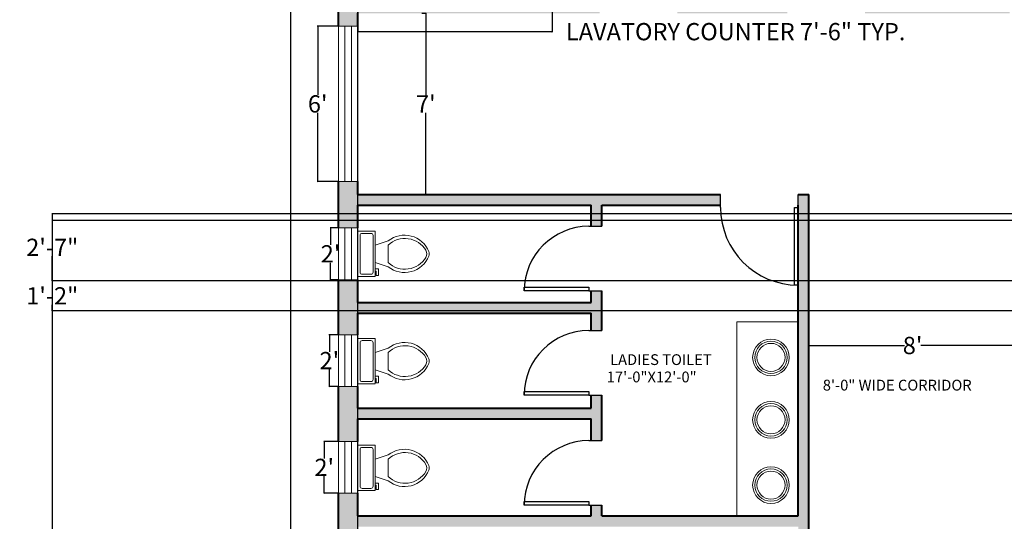
# Model space of a CAD drawing. Units: inches. Extents: x -405 to 940, y 226 to 2032.
# Tile 5 of 10: x -405 to 51, y 1458 to 1691. Entities that reach past the tile are written whole.
import ezdxf

# ---------------------------------------------------------------- set-up
doc = ezdxf.new("R2010")
doc.units = ezdxf.units.IN
doc.header["$MEASUREMENT"] = 0
doc.linetypes.add('ACAD_ISO02W100', pattern=[15, 12, -3])
for name, color, linetype, lineweight in [('A-ANNO-DIMS', 120, 'Continuous', 18), ('A-AREA-IDEN', 32, 'Continuous', 18), ('A-FLOR-FIXT', 175, 'Continuous', 18), ('A-GLAZ-HIDN', 1, 'ACAD_ISO02W100', 18), ('A-WALL-PATT', 8, 'Continuous', 13), ('door', 6, 'Continuous', 25), ('wall', 3, 'Continuous', 40), ('window', 1, 'Continuous', 18)]:
    doc.layers.add(name, color=color, linetype=linetype, lineweight=lineweight)
doc.styles.get("Standard").update_dxf_attribs({"font": 'arial.ttf'})
doc.dimstyles.get("Standard").update_dxf_attribs({"dimtxt": 8, "dimasz": 0.18, "dimexe": 0.18, "dimexo": 0.0625, "dimgap": 0.09, "dimtad": 0, "dimtih": 1, "dimtoh": 1, "dimdec": 0, "dimzin": 0, "dimdsep": 46, "dimlunit": 3, "dimtxsty": 'Standard', "dimblk": 'OBLIQUE', "dimcen": 0.09, "dimadec": 0, "dimazin": 0, "dimtfac": 1, "dimtdec": 0, "dimtofl": 0, "dimtmove": 0, "dimatfit": 3, "dimfxl": 1, "dimtolj": 1, "dimtzin": 0, "dimarcsym": 0})

# ---------------------------------------------------------------- blocks, each defined once
blk = doc.blocks.new('*U3')
for p, q in [((0, 0), (0, -6)), ((30, 0), (30, -6))]:
    blk.add_line(p, q)
blk.add_lwpolyline([(0, 0), (0, 30), (1.75, 30), (1.75, 0)], close=True)
blk.add_arc((0, 0), 30, 0, 90)
blk = doc.blocks.new('*U4')
for p, q in [((0, 0), (0, -6)), ((36, 0), (36, -6))]:
    blk.add_line(p, q)
blk.add_lwpolyline([(0, 0), (0, 36), (1.75, 36), (1.75, 0)], close=True)
blk.add_arc((0, 0), 36, 0, 90)
blk = doc.blocks.new('*U6')
for p, q in [((9.5, -6), (9.5, -2)), ((-10, -8.5), (-8, -8.5)), ((-10, -9.5), (-10, -8.5)), ((-8, -8.5), (-8, -8)), ((-7, -8), (-7, -9.5)), ((-4, -8), (-6, -14)), ((4, -8), (6, -14)), ((-7, -9.5), (-10, -9.5)), ((4, -14), (-4, -14))]:
    blk.add_line(p, q)
blk.add_lwpolyline([(10.5, -8), (10.5, 0), (-10.5, 0), (-10.5, -8)], close=True)
for points in [[(-9.5, -2), (-9.5, -6)], [(8.5, -1), (-8.5, -1)], [(-8.5, -7), (8.5, -7)]]:
    blk.add_lwpolyline(points)
for centre, radius, start, end in [((-8.62, -1.88), 0.884, 81.8699, 188.1301), ((8.62, -1.88), 0.884, 351.8699, 98.1301), ((-8.62, -6.12), 0.884, 171.8699, 278.1301), ((8.62, -6.12), 0.884, 261.8699, 8.1301), ((3.52, -21.58), 12.17, 141.4691, 247.9714), ((4.2, -21.82), 11.33, 136.3677, 238.9468), ((-3.52, -21.58), 12.17, 292.0284, 38.5307), ((-4.2, -21.82), 11.33, 301.053, 43.6321), ((0, -27.88), 4, 245.7318, 294.2682), ((0, -29), 4, 254.8605, 285.1395)]:
    blk.add_arc(centre, radius, start, end)
blk = doc.blocks.new('_Oblique')
at = {"color": 0, "linetype": 'ByBlock', "lineweight": -2}
blk.add_line((-0.5, -0.5), (0.5, 0.5), dxfattribs=at)
blk = doc.blocks.new('*D40')
at = {"layer": 'A-ANNO-DIMS', "color": 0, "lineweight": -2, "transparency": 16777216}
for p, q in [((-39.23, 1543.59), (-39.23, 1539.64)), ((56.77, 1543.59), (56.77, 1539.64)), ((-39.23, 1539.82), (4.99, 1539.82)), ((56.77, 1539.82), (12.54, 1539.82))]:
    blk.add_line(p, q, dxfattribs=at)
at = {"layer": 'Defpoints', "color": 0, "transparency": 16777216}
for p in [(-39.23, 1543.65), (56.77, 1543.65), (56.77, 1539.82)]:
    blk.add_point(p, dxfattribs=at)
at = {"layer": 'A-ANNO-DIMS', "color": 0, "lineweight": -2, "transparency": 16777216, "xscale": 0.18, "yscale": 0.18, "zscale": 0.18, "rotation": 180}
blk.add_blockref('_Oblique', (-39.23, 1539.82), dxfattribs=at)
at = {"layer": 'A-ANNO-DIMS', "color": 0, "lineweight": -2, "transparency": 16777216, "xscale": 0.18, "yscale": 0.18, "zscale": 0.18}
blk.add_blockref('_Oblique', (56.77, 1539.82), dxfattribs=at)
at = {"layer": 'A-ANNO-DIMS', "color": 0, "transparency": 16777216, "insert": (8.77, 1539.82), "char_height": 8, "attachment_point": 5}
blk.add_mtext("\\A1;8'", dxfattribs=at)
blk = doc.blocks.new('*D44')
at = {"layer": 'A-ANNO-DIMS', "color": 0, "lineweight": -2, "transparency": 16777216}
for p, q in [((-257.29, 1887.81), (-279.61, 1887.81)), ((-279.43, 1887.81), (-279.43, 1210.99)), ((-279.43, 525.81), (-279.43, 1202.63)), ((-257.29, 525.81), (-279.61, 525.81))]:
    blk.add_line(p, q, dxfattribs=at)
at = {"layer": 'Defpoints', "color": 0, "transparency": 16777216}
for p in [(-257.23, 1887.81), (-279.43, 525.81), (-257.23, 525.81)]:
    blk.add_point(p, dxfattribs=at)
at = {"layer": 'A-ANNO-DIMS', "color": 0, "lineweight": -2, "transparency": 16777216, "xscale": 0.18, "yscale": 0.18, "zscale": 0.18}
for p, rotation in [((-279.43, 1887.81), 90), ((-279.43, 525.81), 270)]:
    blk.add_blockref('_Oblique', p, dxfattribs=dict(at, rotation=rotation))
at = {"layer": 'A-ANNO-DIMS', "color": 0, "transparency": 16777216, "insert": (-279.43, 1206.81), "char_height": 8, "attachment_point": 5}
blk.add_mtext('\\A1;113\'-6"', dxfattribs=at)
blk = doc.blocks.new('*D56')
at = {"layer": 'A-ANNO-DIMS', "color": 0, "lineweight": -2, "transparency": 16777216}
for p, q in [((-257.29, 1495.31), (-264.03, 1495.31)), ((-263.85, 1495.31), (-263.85, 1487.42)), ((-263.85, 1471.31), (-263.85, 1479.2)), ((-257.29, 1471.31), (-264.03, 1471.31))]:
    blk.add_line(p, q, dxfattribs=at)
at = {"layer": 'Defpoints', "color": 0, "transparency": 16777216}
for p in [(-263.85, 1495.31), (-257.23, 1495.31), (-257.23, 1471.31)]:
    blk.add_point(p, dxfattribs=at)
at = {"layer": 'A-ANNO-DIMS', "color": 0, "lineweight": -2, "transparency": 16777216, "xscale": 0.18, "yscale": 0.18, "zscale": 0.18}
for p, rotation in [((-263.85, 1495.31), 90), ((-263.85, 1471.31), 270)]:
    blk.add_blockref('_Oblique', p, dxfattribs=dict(at, rotation=rotation))
at = {"layer": 'A-ANNO-DIMS', "color": 0, "transparency": 16777216, "insert": (-263.85, 1483.31), "char_height": 8, "attachment_point": 5}
blk.add_mtext("\\A1;2'", dxfattribs=at)
blk = doc.blocks.new('*D57')
at = {"layer": 'A-ANNO-DIMS', "color": 0, "lineweight": -2, "transparency": 16777216}
for p, q in [((-257.29, 1544.81), (-261.65, 1544.81)), ((-261.47, 1544.81), (-261.47, 1536.92)), ((-261.47, 1520.81), (-261.47, 1528.7)), ((-257.29, 1520.81), (-261.65, 1520.81))]:
    blk.add_line(p, q, dxfattribs=at)
at = {"layer": 'Defpoints', "color": 0, "transparency": 16777216}
for p in [(-261.47, 1544.81), (-257.23, 1544.81), (-257.23, 1520.81)]:
    blk.add_point(p, dxfattribs=at)
at = {"layer": 'A-ANNO-DIMS', "color": 0, "lineweight": -2, "transparency": 16777216, "xscale": 0.18, "yscale": 0.18, "zscale": 0.18}
for p, rotation in [((-261.47, 1544.81), 90), ((-261.47, 1520.81), 270)]:
    blk.add_blockref('_Oblique', p, dxfattribs=dict(at, rotation=rotation))
at = {"layer": 'A-ANNO-DIMS', "color": 0, "transparency": 16777216, "insert": (-261.47, 1532.81), "char_height": 8, "attachment_point": 5}
blk.add_mtext("\\A1;2'", dxfattribs=at)
blk = doc.blocks.new('*D58')
at = {"layer": 'A-ANNO-DIMS', "color": 0, "lineweight": -2, "transparency": 16777216}
for p, q in [((-257.29, 1594.31), (-261.11, 1594.31)), ((-260.93, 1594.31), (-260.93, 1586.42)), ((-260.93, 1570.31), (-260.93, 1578.2)), ((-257.29, 1570.31), (-261.11, 1570.31))]:
    blk.add_line(p, q, dxfattribs=at)
at = {"layer": 'Defpoints', "color": 0, "transparency": 16777216}
for p in [(-260.93, 1594.31), (-257.23, 1594.31), (-257.23, 1570.31)]:
    blk.add_point(p, dxfattribs=at)
at = {"layer": 'A-ANNO-DIMS', "color": 0, "lineweight": -2, "transparency": 16777216, "xscale": 0.18, "yscale": 0.18, "zscale": 0.18}
for p, rotation in [((-260.93, 1594.31), 90), ((-260.93, 1570.31), 270)]:
    blk.add_blockref('_Oblique', p, dxfattribs=dict(at, rotation=rotation))
at = {"layer": 'A-ANNO-DIMS', "color": 0, "transparency": 16777216, "insert": (-260.93, 1582.31), "char_height": 8, "attachment_point": 5}
blk.add_mtext("\\A1;2'", dxfattribs=at)
blk = doc.blocks.new('*D59')
at = {"layer": 'A-ANNO-DIMS', "color": 0, "lineweight": -2, "transparency": 16777216}
for p, q in [((-218.67, 1693.81), (-216.61, 1693.81)), ((-216.79, 1693.81), (-216.79, 1655.9)), ((-216.79, 1609.81), (-216.79, 1647.72)), ((-218.67, 1609.81), (-216.61, 1609.81))]:
    blk.add_line(p, q, dxfattribs=at)
at = {"layer": 'Defpoints', "color": 0, "transparency": 16777216}
for p in [(-218.73, 1693.81), (-218.73, 1609.81), (-216.79, 1609.81)]:
    blk.add_point(p, dxfattribs=at)
at = {"layer": 'A-ANNO-DIMS', "color": 0, "lineweight": -2, "transparency": 16777216, "xscale": 0.18, "yscale": 0.18, "zscale": 0.18}
for p, rotation in [((-216.79, 1693.81), 90), ((-216.79, 1609.81), 270)]:
    blk.add_blockref('_Oblique', p, dxfattribs=dict(at, rotation=rotation))
at = {"layer": 'A-ANNO-DIMS', "color": 0, "transparency": 16777216, "insert": (-216.79, 1651.81), "char_height": 8, "attachment_point": 5}
blk.add_mtext("\\A1;7'", dxfattribs=at)
blk = doc.blocks.new('*D60')
at = {"layer": 'A-ANNO-DIMS', "color": 0, "lineweight": -2, "transparency": 16777216}
for p, q in [((-257.29, 1687.81), (-267.07, 1687.81)), ((-266.89, 1687.81), (-266.89, 1655.98)), ((-266.89, 1615.81), (-266.89, 1647.64)), ((-257.29, 1615.81), (-267.07, 1615.81))]:
    blk.add_line(p, q, dxfattribs=at)
at = {"layer": 'Defpoints', "color": 0, "transparency": 16777216}
for p in [(-266.89, 1687.81), (-257.23, 1687.81), (-257.23, 1615.81)]:
    blk.add_point(p, dxfattribs=at)
at = {"layer": 'A-ANNO-DIMS', "color": 0, "lineweight": -2, "transparency": 16777216, "xscale": 0.18, "yscale": 0.18, "zscale": 0.18}
for p, rotation in [((-266.89, 1687.81), 90), ((-266.89, 1615.81), 270)]:
    blk.add_blockref('_Oblique', p, dxfattribs=dict(at, rotation=rotation))
at = {"layer": 'A-ANNO-DIMS', "color": 0, "transparency": 16777216, "insert": (-266.89, 1651.81), "char_height": 8, "attachment_point": 5}
blk.add_mtext("\\A1;6'", dxfattribs=at)
blk = doc.blocks.new('LAVATORY-COUNTER-TRIPLE')
for p, q in [((0, 28.51), (89.99, 28.51)), ((89.99, 28.51), (89.99, 0))]:
    blk.add_line(p, q)
for centre, radius in [((14.28, 12.62), 8.5), ((14.28, 12.62), 7.5), ((14.28, 12.62), 6.5), ((44.55, 12.62), 8.5), ((44.55, 12.62), 7.5), ((44.55, 12.62), 6.5), ((73.49, 12.62), 8.5), ((73.49, 12.62), 7.5), ((73.49, 12.62), 6.5)]:
    blk.add_circle(centre, radius)
blk = doc.blocks.new('WIN-PANE-24IN')
for p, q in [((0, 3), (24, 3)), ((0, 0), (24, 0))]:
    blk.add_line(p, q)
blk = doc.blocks.new('WIN-PANE-72IN')
for p, q in [((0, 3), (72, 3)), ((0, 0), (72, 0))]:
    blk.add_line(p, q)
blk = doc.blocks.new('*D93')
at = {"layer": 'A-ANNO-DIMS', "color": 0, "lineweight": -2, "transparency": 16777216}
for p, q in [((-248.23, 1698.75), (-248.23, 1685.13)), ((-158.24, 1698.75), (-158.24, 1685.13)), ((-248.23, 1685.31), (-158.24, 1685.31)), ((-158.24, 1685.31), (-158.06, 1685.31))]:
    blk.add_line(p, q, dxfattribs=at)
at = {"layer": 'Defpoints', "color": 0, "transparency": 16777216}
for p in [(-248.23, 1698.81), (-158.24, 1698.81), (-158.24, 1685.31)]:
    blk.add_point(p, dxfattribs=at)
at = {"layer": 'A-ANNO-DIMS', "color": 0, "lineweight": -2, "transparency": 16777216, "xscale": 0.18, "yscale": 0.18, "zscale": 0.18, "rotation": 180}
blk.add_blockref('_Oblique', (-248.23, 1685.31), dxfattribs=at)
at = {"layer": 'A-ANNO-DIMS', "color": 0, "lineweight": -2, "transparency": 16777216, "xscale": 0.18, "yscale": 0.18, "zscale": 0.18}
blk.add_blockref('_Oblique', (-158.24, 1685.31), dxfattribs=at)
at = {"layer": 'A-ANNO-DIMS', "color": 0, "transparency": 16777216, "insert": (-73.22, 1685.31), "char_height": 8, "attachment_point": 5}
blk.add_mtext('\\A1;LAVATORY COUNTER 7\'-6" TYP.', dxfattribs=at)
blk = doc.blocks.new('*D100')
at = {"layer": 'A-ANNO-DIMS', "color": 0, "lineweight": -2, "transparency": 16777216}
for p, q in [((626.71, 1569.84), (-390.06, 1569.84)), ((-389.88, 1569.84), (-389.88, 1566.93)), ((626.71, 1555.81), (-390.06, 1555.81)), ((-389.88, 1555.81), (-389.88, 1558.72))]:
    blk.add_line(p, q, dxfattribs=at)
at = {"layer": 'Defpoints', "color": 0, "transparency": 16777216}
for p in [(626.77, 1569.84), (-389.88, 1555.81), (626.77, 1555.81)]:
    blk.add_point(p, dxfattribs=at)
at = {"layer": 'A-ANNO-DIMS', "color": 0, "lineweight": -2, "transparency": 16777216, "xscale": 0.18, "yscale": 0.18, "zscale": 0.18}
for p, rotation in [((-389.88, 1569.84), 90), ((-389.88, 1555.81), 270)]:
    blk.add_blockref('_Oblique', p, dxfattribs=dict(at, rotation=rotation))
at = {"layer": 'A-ANNO-DIMS', "color": 0, "transparency": 16777216, "insert": (-389.88, 1562.83), "char_height": 8, "attachment_point": 5}
blk.add_mtext('\\A1;1\'-2"', dxfattribs=at)
blk = doc.blocks.new('*D105')
at = {"layer": 'A-ANNO-DIMS', "color": 0, "lineweight": -2, "transparency": 16777216}
for p, q in [((602.71, 1600.81), (-390.06, 1600.81)), ((-389.88, 1600.81), (-389.88, 1589.43)), ((-389.88, 1569.84), (-389.88, 1581.22)), ((626.71, 1569.84), (-390.06, 1569.84))]:
    blk.add_line(p, q, dxfattribs=at)
at = {"layer": 'Defpoints', "color": 0, "transparency": 16777216}
for p in [(602.77, 1600.81), (-389.88, 1569.84), (626.77, 1569.84)]:
    blk.add_point(p, dxfattribs=at)
at = {"layer": 'A-ANNO-DIMS', "color": 0, "lineweight": -2, "transparency": 16777216, "xscale": 0.18, "yscale": 0.18, "zscale": 0.18}
for p, rotation in [((-389.88, 1600.81), 90), ((-389.88, 1569.84), 270)]:
    blk.add_blockref('_Oblique', p, dxfattribs=dict(at, rotation=rotation))
at = {"layer": 'A-ANNO-DIMS', "color": 0, "transparency": 16777216, "insert": (-389.88, 1585.33), "char_height": 8, "attachment_point": 5}
blk.add_mtext('\\A1;2\'-7"', dxfattribs=at)
blk = doc.blocks.new('*D107')
at = {"layer": 'A-ANNO-DIMS', "color": 0, "lineweight": -2, "transparency": 16777216}
for p, q in [((501.71, 1597.81), (-390.06, 1597.81)), ((-389.88, 1597.81), (-389.88, 1228.98)), ((-389.88, 851.81), (-389.88, 1220.64)), ((501.71, 851.81), (-390.06, 851.81))]:
    blk.add_line(p, q, dxfattribs=at)
at = {"layer": 'Defpoints', "color": 0, "transparency": 16777216}
for p in [(-389.88, 1597.81), (501.77, 1597.81), (501.77, 851.81)]:
    blk.add_point(p, dxfattribs=at)
at = {"layer": 'A-ANNO-DIMS', "color": 0, "lineweight": -2, "transparency": 16777216, "xscale": 0.18, "yscale": 0.18, "zscale": 0.18}
for p, rotation in [((-389.88, 1597.81), 90), ((-389.88, 851.81), 270)]:
    blk.add_blockref('_Oblique', p, dxfattribs=dict(at, rotation=rotation))
at = {"layer": 'A-ANNO-DIMS', "color": 0, "transparency": 16777216, "insert": (-389.88, 1224.81), "char_height": 8, "attachment_point": 5}
blk.add_mtext('\\A1;62\'-2"', dxfattribs=at)
blk = doc.blocks.new('*D109')
at = {"layer": 'A-ANNO-DIMS', "color": 0, "lineweight": -2, "transparency": 16777216}
for p, q in [((-248.23, 750.87), (-248.23, 2020.64)), ((-248.23, 2020.46), (-49.06, 2020.46)), ((177.77, 2020.46), (-21.4, 2020.46)), ((177.77, 750.87), (177.77, 2020.64))]:
    blk.add_line(p, q, dxfattribs=at)
at = {"layer": 'Defpoints', "color": 0, "transparency": 16777216}
for p in [(177.77, 2020.46), (-248.23, 750.81), (177.77, 750.81)]:
    blk.add_point(p, dxfattribs=at)
at = {"layer": 'A-ANNO-DIMS', "color": 0, "lineweight": -2, "transparency": 16777216, "xscale": 0.18, "yscale": 0.18, "zscale": 0.18, "rotation": 180}
blk.add_blockref('_Oblique', (-248.23, 2020.46), dxfattribs=at)
at = {"layer": 'A-ANNO-DIMS', "color": 0, "lineweight": -2, "transparency": 16777216, "xscale": 0.18, "yscale": 0.18, "zscale": 0.18}
blk.add_blockref('_Oblique', (177.77, 2020.46), dxfattribs=at)
at = {"layer": 'A-ANNO-DIMS', "color": 0, "transparency": 16777216, "insert": (-35.23, 2020.46), "char_height": 8, "attachment_point": 5}
blk.add_mtext('\\A1;35\'-6"', dxfattribs=at)

msp = doc.modelspace()

# ---------------------------------------------------------------- hatches: boundary and pattern name
at = {"layer": 'A-WALL-PATT'}
h = msp.add_hatch(dxfattribs=at)
h.set_pattern_fill('AR-HBONE', color=256)
h.set_pattern_definition([(45, (599.8442, 904.9158), (0, 5.656854), [12, -4]), (135, (602.6726, 907.744), (4e-16, 5.656854), [12, -4])])
h.paths.add_polyline_path([(-248.23, 1045.81), (-257.23, 1045.81), (-257.23, 964.81), (-248.23, 964.81)], flags=17)
h.paths.add_polyline_path([(-248.23, 851.81), (-39.23, 851.81), (-39.23, 856.81), (-44.23, 856.81), (-248.23, 856.81), (-248.23, 892.81), (-257.23, 892.81), (-257.23, 839.81), (-248.23, 839.81)])
h.paths.add_polyline_path([(-248.23, 750.81), (124.74, 750.81), (124.74, 751.73), (124.74, 755.81), (-248.23, 755.81), (-248.23, 767.81), (-257.23, 767.81), (-257.23, 726.81), (-248.23, 726.81)])
h.paths.add_polyline_path([(-248.23, 654.81), (-257.23, 654.81), (-257.23, 630.81), (-248.23, 630.81)])
h.paths.add_polyline_path([(-180.23, 534.81), (-248.23, 534.81), (-248.23, 558.81), (-257.23, 558.81), (-257.23, 525.81), (-180.23, 525.81)])
h.paths.add_polyline_path([(-69.23, 534.81), (-108.23, 534.81), (-108.23, 525.81), (-69.23, 525.81)])
h.paths.add_polyline_path([(35.77, 534.81), (2.77, 534.81), (2.77, 525.81), (35.77, 525.81)])
h.paths.add_polyline_path([(182.77, 755.81), (160.74, 755.81), (160.74, 750.81), (177.77, 750.81), (177.77, 534.81), (107.77, 534.81), (107.77, 525.81), (182.77, 525.81)])
h.paths.add_polyline_path([(-39.23, 1609.81), (-44.23, 1609.81), (-44.23, 1604.81), (-44.23, 1460.81), (-135.23, 1460.81), (-135.23, 1465.73), (-140.23, 1465.73), (-140.23, 1460.81), (-248.23, 1460.81), (-248.23, 1471.31), (-257.23, 1471.31), (-257.23, 1419.81), (-248.23, 1419.81), (-248.23, 1455.81), (-44.23, 1455.81), (-44.23, 1194.81), (-39.23, 1194.81)])
h.paths.add_polyline_path([(-248.23, 1520.81), (-257.23, 1520.81), (-257.23, 1495.31), (-248.23, 1495.31), (-248.23, 1505.81), (-140.23, 1505.81), (-140.23, 1495.73), (-135.23, 1495.73), (-135.23, 1516.79), (-140.23, 1516.79), (-140.23, 1510.81), (-248.23, 1510.81)], flags=17)
h.paths.add_polyline_path([(-248.23, 1570.31), (-257.23, 1570.31), (-257.23, 1544.81), (-248.23, 1544.81), (-248.23, 1554.81), (-140.23, 1554.81), (-140.23, 1546.79), (-135.23, 1546.79), (-135.23, 1565.08), (-140.23, 1565.08), (-140.23, 1559.81), (-248.23, 1559.81)], flags=17)
h.paths.add_polyline_path([(-248.23, 1615.81), (-257.23, 1615.81), (-257.23, 1594.31), (-248.23, 1594.31), (-248.23, 1604.81), (-140.23, 1604.81), (-140.23, 1595.08), (-135.23, 1595.08), (-135.23, 1604.81), (-80.23, 1604.81), (-80.23, 1609.81), (-248.23, 1609.81)])
h.paths.add_polyline_path([(-248.23, 1783.81), (-235.46, 1783.81), (-235.46, 1788.81), (-248.23, 1788.81), (-248.23, 1878.81), (-237.73, 1878.81), (-237.73, 1887.81), (-257.23, 1887.81), (-257.23, 1687.81), (-248.23, 1687.81), (-248.23, 1693.81), (-136.23, 1693.81), (-136.23, 1698.81), (-248.23, 1698.81)])
h.paths.add_polyline_path([(-188.23, 1887.81), (-213.73, 1887.81), (-213.73, 1878.81), (-203.23, 1878.81), (-203.23, 1788.81), (-205.46, 1788.81), (-205.46, 1783.81), (-186.39, 1783.81), (-186.39, 1788.81), (-198.23, 1788.81), (-198.23, 1878.81), (-188.23, 1878.81)])
h.paths.add_polyline_path([(-139.23, 1887.81), (-164.23, 1887.81), (-164.23, 1878.81), (-154.23, 1878.81), (-154.23, 1788.81), (-156.39, 1788.81), (-156.39, 1783.81), (-138.25, 1783.81), (-138.25, 1788.81), (-149.23, 1788.81), (-149.23, 1878.81), (-139.23, 1878.81)])
h.paths.add_polyline_path([(-89.23, 1887.81), (-115.23, 1887.81), (-115.23, 1878.81), (-105.23, 1878.81), (-105.23, 1788.81), (-108.25, 1788.81), (-108.25, 1783.81), (-86.45, 1783.81), (-86.45, 1788.81), (-100.23, 1788.81), (-100.23, 1878.81), (-89.23, 1878.81)])
h.paths.add_polyline_path([(-36.23, 1887.81), (-65.23, 1887.81), (-65.23, 1878.81), (-54.23, 1878.81), (-54.23, 1788.81), (-56.45, 1788.81), (-56.45, 1783.81), (-54.23, 1783.81), (-54.23, 1698.81), (-100.23, 1698.81), (-100.23, 1693.81), (-49.23, 1693.81), (-49.23, 1698.81), (-49.23, 1878.81), (-36.23, 1878.81)])
h.paths.add_polyline_path([(89.77, 1887.81), (35.77, 1887.81), (35.77, 1878.81), (48.77, 1878.81), (48.77, 1698.81), (-13.23, 1698.81), (-13.23, 1693.81), (53.77, 1693.81), (53.77, 1698.81), (53.77, 1878.81), (89.77, 1878.81)])
h.paths.add_polyline_path([(255.27, 1887.81), (161.77, 1887.81), (161.77, 1878.81), (197.77, 1878.81), (197.77, 1698.81), (89.77, 1698.81), (89.77, 1693.81), (202.77, 1693.81), (202.77, 1698.81), (202.77, 1878.81), (255.27, 1878.81)])
h.paths.add_polyline_path([(375.27, 1887.81), (327.27, 1887.81), (327.27, 1878.81), (375.27, 1878.81)], flags=17)
h.paths.add_polyline_path([(815.77, 1887.81), (447.27, 1887.81), (447.27, 1878.81), (499.77, 1878.81), (499.77, 1698.81), (238.77, 1698.81), (238.77, 1693.81), (504.77, 1693.81), (504.77, 1878.81), (633.77, 1878.81), (633.77, 1646.81), (597.77, 1646.81), (597.77, 1641.81), (602.77, 1641.81), (638.77, 1641.81), (638.77, 1878.81), (806.77, 1878.81), (806.77, 1838.31), (815.77, 1838.31)])
h.paths.add_polyline_path([(815.77, 1766.31), (806.77, 1766.31), (806.77, 1718.31), (815.77, 1718.31)], flags=17)
h.paths.add_polyline_path([(815.77, 1356.31), (806.77, 1356.31), (806.77, 1303.81), (602.77, 1303.81), (597.77, 1303.81), (597.77, 1037.81), (602.77, 1037.81), (602.77, 1298.81), (806.77, 1298.81), (806.77, 1246.31), (815.77, 1246.31)])
h.paths.add_polyline_path([(815.77, 1174.31), (806.77, 1174.31), (806.77, 1126.31), (815.77, 1126.31)], flags=17)
h.paths.add_polyline_path([(815.77, 1054.31), (806.77, 1054.31), (806.77, 1001.81), (796.08, 1001.81), (796.08, 1001.75), (780.86, 1001.75), (602.77, 1001.81), (597.77, 1001.81), (597.77, 892.81), (602.77, 892.81), (602.77, 996.81), (806.77, 996.81), (806.77, 962.81), (815.77, 962.81)])
h.paths.add_polyline_path([(403.77, 534.81), (379.77, 534.81), (379.77, 525.81), (403.77, 525.81)])
h.paths.add_polyline_path([(-39.23, 1158.81), (-44.23, 1158.81), (-248.23, 1158.81), (-248.23, 1194.81), (-257.23, 1194.81), (-257.23, 1117.81), (-248.23, 1117.81), (-248.23, 1153.81), (-44.23, 1153.81), (-44.23, 892.81), (-39.23, 892.81)])
h.paths.add_polyline_path([(-248.23, 1347.81), (-257.23, 1347.81), (-257.23, 1275.81), (-248.23, 1275.81)], flags=17)
h.paths.add_polyline_path([(815.77, 1476.31), (806.77, 1476.31), (806.77, 1428.31), (815.77, 1428.31)], flags=17)
h.paths.add_polyline_path([(815.77, 1646.31), (806.77, 1646.31), (806.77, 1638.65), (806.77, 1605.81), (597.77, 1605.81), (597.77, 1339.81), (602.77, 1339.81), (602.77, 1600.81), (806.77, 1600.81), (806.77, 1548.31), (815.77, 1548.31)])

# ---------------------------------------------------------------- linework, layer by layer
at = {"layer": 'A-GLAZ-HIDN'}
for p, q in [((-248.23, 1687.81), (-257.23, 1687.81)), ((-248.23, 1615.81), (-257.23, 1615.81)), ((-248.23, 1594.31), (-257.23, 1594.31)), ((-248.23, 1570.31), (-257.23, 1570.31)), ((-248.23, 1544.81), (-257.23, 1544.81)), ((-248.23, 1520.81), (-257.23, 1520.81)), ((-248.23, 1495.31), (-257.23, 1495.31)), ((-248.23, 1471.31), (-257.23, 1471.31))]:
    msp.add_line(p, q, dxfattribs=at)
at = {"layer": 'door'}
for p, q in [((-80.23, 1604.81), (-80.23, 1609.81)), ((-44.23, 1604.81), (-44.23, 1609.81)), ((-140.23, 1595.08), (-135.23, 1595.08)), ((-140.23, 1565.08), (-135.23, 1565.08)), ((-140.23, 1546.79), (-135.23, 1546.79)), ((-140.23, 1516.79), (-135.23, 1516.79)), ((-140.23, 1495.73), (-135.23, 1495.73)), ((-140.23, 1465.73), (-135.23, 1465.73))]:
    msp.add_line(p, q, dxfattribs=at)
at = {"layer": 'wall'}
for p, q in [((-257.23, 1687.81), (-257.23, 1887.81)), ((-248.23, 1687.81), (-248.23, 1693.81)), ((-257.23, 1594.31), (-257.23, 1615.81)), ((-248.23, 1609.81), (-248.23, 1615.81)), ((-248.23, 1609.81), (-80.23, 1609.81)), ((-44.23, 1609.81), (-39.23, 1609.81)), ((-39.23, 1194.81), (-39.23, 1609.81)), ((-248.23, 1604.81), (-140.23, 1604.81)), ((-248.23, 1594.31), (-248.23, 1604.81)), ((-140.23, 1595.08), (-140.23, 1604.81)), ((-135.23, 1604.81), (-80.23, 1604.81)), ((-135.23, 1595.08), (-135.23, 1604.81)), ((-44.23, 1460.81), (-44.23, 1604.81)), ((-257.23, 1544.81), (-257.23, 1570.31)), ((-248.23, 1559.81), (-248.23, 1570.31)), ((-140.23, 1559.81), (-140.23, 1565.08)), ((-135.23, 1546.79), (-135.23, 1565.08)), ((-248.23, 1559.81), (-140.23, 1559.81)), ((-248.23, 1554.81), (-140.23, 1554.81)), ((-248.23, 1544.81), (-248.23, 1554.81)), ((-140.23, 1546.79), (-140.23, 1554.81)), ((-257.23, 1495.31), (-257.23, 1520.81)), ((-248.23, 1510.81), (-248.23, 1520.81)), ((-140.23, 1510.81), (-140.23, 1516.79)), ((-135.23, 1495.73), (-135.23, 1516.79)), ((-248.23, 1510.81), (-140.23, 1510.81)), ((-248.23, 1505.81), (-140.23, 1505.81)), ((-248.23, 1495.31), (-248.23, 1505.81)), ((-140.23, 1495.73), (-140.23, 1505.81)), ((-257.23, 1419.81), (-257.23, 1471.31)), ((-248.23, 1460.81), (-248.23, 1471.31)), ((-140.23, 1460.81), (-140.23, 1465.73)), ((-135.23, 1460.81), (-135.23, 1465.73)), ((-248.23, 1460.81), (-140.23, 1460.81)), ((-135.23, 1460.81), (-44.23, 1460.81))]:
    msp.add_line(p, q, dxfattribs=at)
at = {"layer": 'window'}
for p, q in [((-257.23, 1615.81), (-257.23, 1687.81)), ((-248.23, 1615.81), (-248.23, 1687.81)), ((-257.23, 1570.31), (-257.23, 1594.31)), ((-248.23, 1570.31), (-248.23, 1594.31)), ((-257.23, 1520.81), (-257.23, 1544.81)), ((-248.23, 1520.81), (-248.23, 1544.81)), ((-257.23, 1471.31), (-257.23, 1495.31)), ((-248.23, 1471.31), (-248.23, 1495.31))]:
    msp.add_line(p, q, dxfattribs=at)

# ---------------------------------------------------------------- block references
at = {"layer": 'A-FLOR-FIXT'}
for name, p, rotation in [('*U6', (-248.23, 1582.31), 90), ('LAVATORY-COUNTER-TRIPLE', (-44.23, 1460.81), 90.00000000000011), ('*U6', (-248.23, 1532.57), 90), ('*U6', (-248.23, 1483.07), 90)]:
    msp.add_blockref(name, p, dxfattribs=dict(at, rotation=rotation))
at = {"layer": 'door'}
for name, p, rotation in [('*U4', (-44.23, 1603.81), 180), ('*U3', (-141.23, 1565.08), 90), ('*U3', (-141.23, 1516.79), 90), ('*U3', (-141.23, 1465.73), 90)]:
    msp.add_blockref(name, p, dxfattribs=dict(at, rotation=rotation))
at = {"layer": 'window'}
for name, p, rotation in [('WIN-PANE-72IN', (-251.23, 1615.81), 90.00000000000003), ('WIN-PANE-24IN', (-254.23, 1594.31), 269.9999999999989), ('WIN-PANE-24IN', (-254.23, 1544.81), 269.9999999999989), ('WIN-PANE-24IN', (-254.23, 1495.31), 269.9999999999989)]:
    msp.add_blockref(name, p, dxfattribs=dict(at, rotation=rotation))

# ---------------------------------------------------------------- texts
at = {"layer": 'A-AREA-IDEN'}
for s, p in [(' LADIES TOILET ', (-132.93, 1530.77)), ('17\'-0"X12\'-0"', (-132.93, 1522.74)), ('8\'-0" WIDE CORRIDOR', (-32.84, 1518.94))]:
    msp.add_text(s, height=5, dxfattribs=at).set_placement(p)

# ---------------------------------------------------------------- dimensions: what is measured, and where the dimension line sits
at = {"layer": 'A-ANNO-DIMS'}
for base, p1, p2, override, picture, middle in [((177.77, 2020.46), (-248.23, 750.81), (177.77, 750.81), {"dimdec": 1, "dimlfac": 1, "dimrnd": 0, "dimzin": 1, "dimdsep": 46, "dimlunit": 4, "dimfrac": 2}, '*D109', (-35.23, 2020.46)), ((56.77, 1539.82), (-39.23, 1543.65), (56.77, 1543.65), {"dimclrd": 0, "dimclre": 0, "dimclrt": 0}, '*D40', (8.77, 1539.82))]:
    dim = msp.add_linear_dim(base=base, p1=p1, p2=p2, dimstyle='Standard', override=override, dxfattribs=at)
    dim.commit()
    dim.dimension.update_dxf_attribs({"geometry": picture, "text_midpoint": middle})
for base, p1, p2, override, picture, middle in [((-279.43, 525.81), (-257.23, 1887.81), (-257.23, 525.81), {"dimclrd": 0, "dimclre": 0, "dimclrt": 0}, '*D44', (-279.43, 1206.81)), ((-216.79, 1609.81), (-218.73, 1693.81), (-218.73, 1609.81), {"dimclrd": 0, "dimclre": 0, "dimclrt": 0}, '*D59', (-216.79, 1651.81)), ((-266.89, 1687.81), (-257.23, 1615.81), (-257.23, 1687.81), {"dimclrd": 0, "dimclre": 0, "dimclrt": 0}, '*D60', (-266.89, 1651.81)), ((-389.88, 1597.81), (501.77, 851.81), (501.77, 1597.81), {"dimdec": 1, "dimlfac": 1, "dimrnd": 0, "dimzin": 1, "dimdsep": 46, "dimlunit": 4, "dimfrac": 2}, '*D107', (-389.88, 1224.81)), ((-389.88, 1569.84), (602.77, 1600.81), (626.77, 1569.84), {"dimdec": 1, "dimlfac": 1, "dimrnd": 0, "dimzin": 1, "dimdsep": 46, "dimlunit": 4, "dimfrac": 2}, '*D105', (-389.88, 1585.33)), ((-260.93, 1594.31), (-257.23, 1570.31), (-257.23, 1594.31), {"dimclrd": 0, "dimclre": 0, "dimclrt": 0}, '*D58', (-260.93, 1582.31)), ((-389.88, 1555.81), (626.77, 1569.84), (626.77, 1555.81), {"dimdec": 1, "dimlfac": 1, "dimrnd": 0, "dimzin": 1, "dimdsep": 46, "dimlunit": 4, "dimfrac": 2}, '*D100', (-389.88, 1562.83)), ((-261.47, 1544.81), (-257.23, 1520.81), (-257.23, 1544.81), {"dimclrd": 0, "dimclre": 0, "dimclrt": 0}, '*D57', (-261.47, 1532.81)), ((-263.85, 1495.31), (-257.23, 1471.31), (-257.23, 1495.31), {"dimclrd": 0, "dimclre": 0, "dimclrt": 0}, '*D56', (-263.85, 1483.31))]:
    dim = msp.add_linear_dim(base=base, p1=p1, p2=p2, angle=90, dimstyle='Standard', override=override, dxfattribs=at)
    dim.commit()
    dim.dimension.update_dxf_attribs({"geometry": picture, "text_midpoint": middle})
dim = msp.add_linear_dim(base=(-158.24, 1685.31), p1=(-248.23, 1698.81), p2=(-158.24, 1698.81), text='LAVATORY COUNTER <> TYP.', dimstyle='Standard', override={"dimdec": 1, "dimlfac": 1, "dimrnd": 0, "dimzin": 1, "dimdsep": 46, "dimlunit": 4, "dimfrac": 2}, dxfattribs=at)
dim.commit()
dim.dimension.update_dxf_attribs({"geometry": '*D93', "text_midpoint": (-73.22, 1685.31)})

doc.saveas('drawing.dxf')
